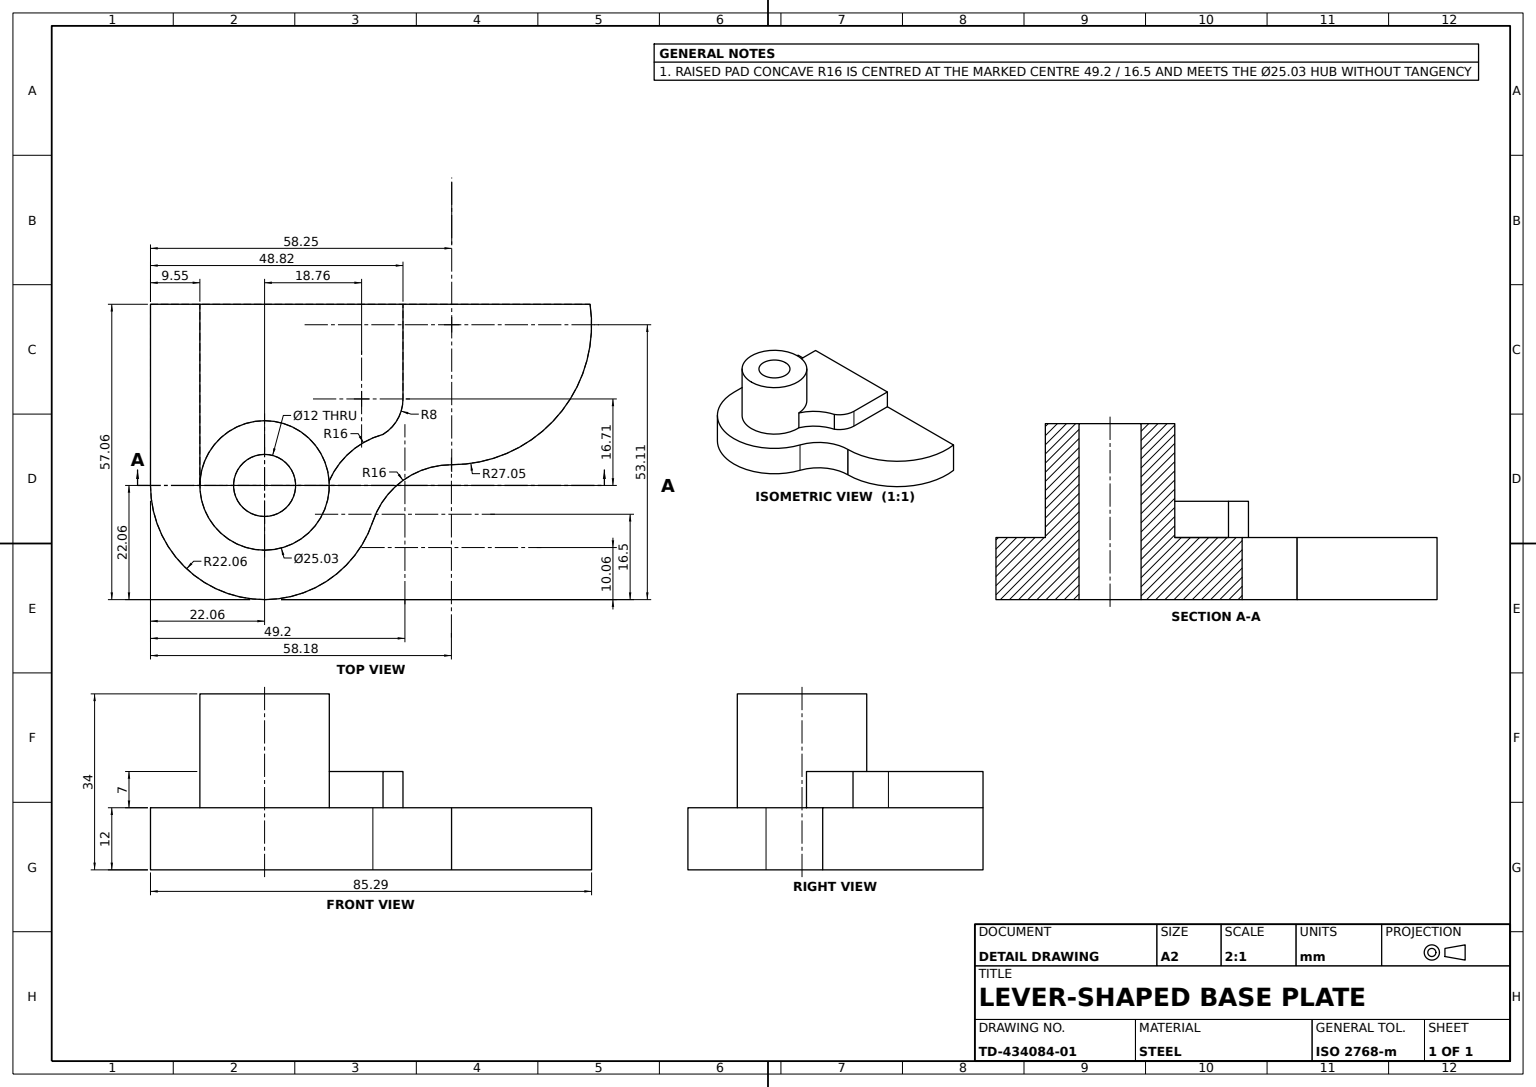
SolidWorks part; units mm, degrees
material "Plain Carbon Steel"
ref_plane "Front Plane" through (0, 0, 0) normal (0, 0, 1) x (1, 0, 0)
ref_plane "Top Plane" through (0, 0, 0) normal (0, 1, 0) x (1, 0, 0)
ref_plane "Right Plane" through (0, 0, 0) normal (1, 0, 0) x (0, 0, -1)
sketch "Base Plate Profile" plane through (0, 0, 0) normal (0, 1, 0) x (1, 0, 0)
  line L0 (-22.063, 0) -> (-22.063, 35)
  line L1 (-22.063, 35) -> (62.937, 35)
  line L4 (36.1825, 4) -> (36.1219, 4)
  arc A0 (-22.063, 0) -> (20.9379, -6.9557) centre (0, 0) ccw
  arc A1 (36.1825, 4) -> (62.937, 35) centre (36.1825, 31.0452) ccw
  arc A2 (36.1219, 4) -> (20.9379, -6.9557) centre (36.1219, -12) ccw
  dimension "D1" = 31
  dimension "D4" = 22.063
  dimension "D5" = 27.0452
  dimension "D6" = 16
  dimension "D2" = 85
  dimension "D3" = 35
extrude "Base Plate" add sketch "Base Plate Profile" along normal blind 12
sketch "Raised Pad Profile" plane through (0, 12, 0) normal (0, 1, 0) x (1, 0, 0)
  line L0 (-12.513, 0) -> (-12.513, 35)
  line L1 (62.937, 35) -> (-22.063, 35) construction
  line L2 (26.76, 16.7083) -> (26.76, 35)
  line L4 (-12.513, 35) -> (26.76, 35)
  line L6 (36.1219, 4) -> (36.1825, 4)
  line L7 (62.937, 35) -> (-22.063, 35)
  line L8 (-22.063, 35) -> (-22.063, 0)
  line L9 (36.1219, 4) -> (36.1825, 4)
  arc A0 (-12.513, 0) -> (12.4831, 0.8639) centre (0, 0) ccw
  arc A1 (12.4831, 0.8639) -> (22.8999, 9.8628) centre (27.1339, -5.5668) cw
  arc A5 (26.76, 16.7083) -> (22.8999, 9.8628) centre (18.76, 16.7083) cw
  arc A6 (36.1219, 4) -> (20.9379, -6.9557) centre (36.1219, -12) ccw
  arc A7 (36.1825, 4) -> (62.937, 35) centre (36.1825, 31.0452) ccw
  arc A8 (-22.063, 0) -> (20.9379, -6.9557) centre (0, 0) ccw
  line M10 (62.937, 35) -> (-22.063, 35)
  dimension "D1" = 25.026
  dimension "D2" = 8
  dimension "D3" = 18.76
  dimension "D6" = 16
  dimension "D4" = 16.7083
  dimension "D5" = 22.8999
  dimension "D7" = 14.6508
  dimension "D8" = 0
extrude "Raised Pad" add sketch "Raised Pad Profile" along normal blind 7 contours A5 L2 L0 A0 A1 M10
sketch "Hub Boss Profile" plane through (0, 19, 0) normal (0, 1, 0) x (1, 0, 0)
  circle A1 centre (0, 0) radius 12.513
  dimension "D1" = 25.026
extrude "Hub Boss" add sketch "Hub Boss Profile" along normal blind 15
sketch "Bore Ø12 Profile" plane through (0, 34, 0) normal (0, 1, 0) x (1, 0, 0)
  circle A0 centre (0, 0) radius 6
  dimension "D1" = 12
extrude "Bore Ø12" cut sketch "Bore Ø12 Profile" against normal blind 68
